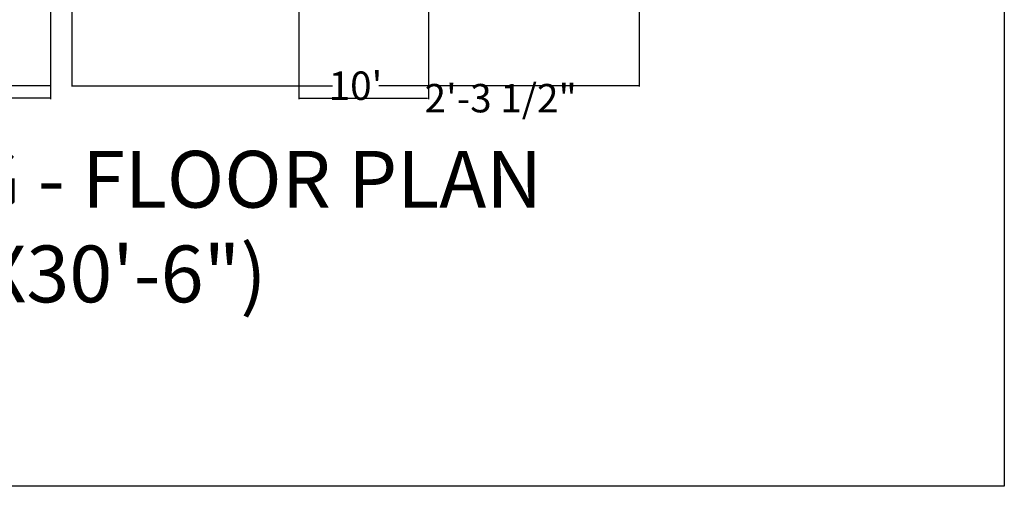
# Model space of a CAD drawing. Units: inches. Extents: x 958 to 1375, y 3152 to 3689.
# Tile 2 of 8: x 1167 to 1375, y 3152 to 3251. Entities that reach past the tile are written whole.
import ezdxf

# ---------------------------------------------------------------- set-up
doc = ezdxf.new("R2010")
doc.units = ezdxf.units.IN
doc.header["$MEASUREMENT"] = 0
doc.layers.add('A-ANNO-DIMS', color=2, linetype='Continuous', lineweight=18)
doc.layers.add('A-ANNO-TTLB', color=7, linetype='Continuous', lineweight=25)
doc.styles.get("Standard").update_dxf_attribs({"font": 'arial.ttf'})
doc.dimstyles.get("Standard").update_dxf_attribs({"dimtxt": 6, "dimasz": 0.18, "dimexe": 0.18, "dimexo": 0.0625, "dimgap": 0.09, "dimtad": 0, "dimtih": 1, "dimtoh": 1, "dimdec": 1, "dimzin": 0, "dimdsep": 46, "dimlunit": 3, "dimtxsty": 'Standard', "dimcen": 0.09, "dimadec": 0, "dimazin": 0, "dimtfac": 1, "dimtdec": 1, "dimtofl": 0, "dimtmove": 0, "dimatfit": 3, "dimfxl": 1, "dimtolj": 1, "dimtzin": 0, "dimarcsym": 0})

# ---------------------------------------------------------------- blocks, each defined once
blk = doc.blocks.new('*D9')
at = {"layer": 'A-ANNO-DIMS', "color": 0, "lineweight": -2, "transparency": 16777216}
for p, q in [((1177.7, 3257.97), (1177.7, 3236.74)), ((1297.7, 3257.97), (1297.7, 3236.74)), ((1177.88, 3236.92), (1232.8, 3236.92)), ((1297.52, 3236.92), (1242.6, 3236.92))]:
    blk.add_line(p, q, dxfattribs=at)
at = {"layer": 'A-ANNO-DIMS', "color": 0, "transparency": 16777216}
for points in [[(1177.88, 3236.95), (1177.88, 3236.89), (1177.7, 3236.92)], [(1297.52, 3236.95), (1297.52, 3236.89), (1297.7, 3236.92)]]:
    blk.add_solid(points, dxfattribs=at)
at = {"layer": 'Defpoints', "color": 0, "transparency": 16777216}
for p in [(1177.7, 3258.03), (1297.7, 3258.03), (1177.7, 3236.92)]:
    blk.add_point(p, dxfattribs=at)
at = {"layer": 'A-ANNO-DIMS', "color": 0, "transparency": 16777216, "insert": (1237.7, 3236.92), "char_height": 6, "attachment_point": 5}
blk.add_mtext("\\A1;10'", dxfattribs=at)
blk = doc.blocks.new('*D10')
at = {"layer": 'A-ANNO-DIMS', "color": 0, "lineweight": -2, "transparency": 16777216}
for p, q in [((1053.2, 3257.97), (1053.2, 3236.74)), ((1173.2, 3257.97), (1173.2, 3236.74)), ((1053.38, 3236.92), (1108.3, 3236.92)), ((1173.02, 3236.92), (1118.1, 3236.92))]:
    blk.add_line(p, q, dxfattribs=at)
at = {"layer": 'A-ANNO-DIMS', "color": 0, "transparency": 16777216}
for points in [[(1053.38, 3236.95), (1053.38, 3236.89), (1053.2, 3236.92)], [(1173.02, 3236.95), (1173.02, 3236.89), (1173.2, 3236.92)]]:
    blk.add_solid(points, dxfattribs=at)
at = {"layer": 'Defpoints', "color": 0, "transparency": 16777216}
for p in [(1053.2, 3258.03), (1173.2, 3258.03), (1173.2, 3236.92)]:
    blk.add_point(p, dxfattribs=at)
at = {"layer": 'A-ANNO-DIMS', "color": 0, "transparency": 16777216, "insert": (1113.2, 3236.92), "char_height": 6, "attachment_point": 5}
blk.add_mtext("\\A1;10'", dxfattribs=at)
blk = doc.blocks.new('*D49')
at = {"layer": 'A-ANNO-DIMS', "color": 0, "lineweight": -2, "transparency": 16777216}
for p, q in [((1225.7, 3386.97), (1225.7, 3234.1)), ((1253.12, 3386.97), (1253.12, 3234.1)), ((1225.88, 3234.28), (1252.94, 3234.28)), ((1253.12, 3234.28), (1253.3, 3234.28))]:
    blk.add_line(p, q, dxfattribs=at)
at = {"layer": 'A-ANNO-DIMS', "color": 0, "transparency": 16777216}
for points in [[(1225.88, 3234.31), (1225.88, 3234.25), (1225.7, 3234.28)], [(1252.94, 3234.31), (1252.94, 3234.25), (1253.12, 3234.28)]]:
    blk.add_solid(points, dxfattribs=at)
at = {"layer": 'Defpoints', "color": 0, "transparency": 16777216}
for p in [(1225.7, 3387.03), (1253.12, 3387.03), (1253.12, 3234.28)]:
    blk.add_point(p, dxfattribs=at)
at = {"layer": 'A-ANNO-DIMS', "color": 0, "transparency": 16777216, "insert": (1268.4, 3234.28), "char_height": 6, "attachment_point": 5}
blk.add_mtext('\\A1;2\'-3 1/2"', dxfattribs=at)
blk = doc.blocks.new('*D60')
at = {"layer": 'A-ANNO-DIMS', "color": 0, "lineweight": -2, "transparency": 16777216}
for p, q in [((1135.31, 3386.97), (1135.31, 3234.1)), ((1173.2, 3386.97), (1173.2, 3234.1)), ((1135.49, 3234.28), (1146.19, 3234.28)), ((1173.02, 3234.28), (1162.32, 3234.28))]:
    blk.add_line(p, q, dxfattribs=at)
at = {"layer": 'A-ANNO-DIMS', "color": 0, "transparency": 16777216}
for points in [[(1135.49, 3234.31), (1135.49, 3234.25), (1135.31, 3234.28)], [(1173.02, 3234.31), (1173.02, 3234.25), (1173.2, 3234.28)]]:
    blk.add_solid(points, dxfattribs=at)
at = {"layer": 'Defpoints', "color": 0, "transparency": 16777216}
for p in [(1135.31, 3387.03), (1173.2, 3387.03), (1173.2, 3234.28)]:
    blk.add_point(p, dxfattribs=at)
at = {"layer": 'A-ANNO-DIMS', "color": 0, "transparency": 16777216, "insert": (1154.25, 3234.28), "char_height": 6, "attachment_point": 5}
blk.add_mtext('\\A1;3\'-2"', dxfattribs=at)

msp = doc.modelspace()

# ---------------------------------------------------------------- linework, layer by layer
at = {"layer": 'A-ANNO-TTLB'}
msp.add_lwpolyline([(958.44, 3689.37), (1374.91, 3689.37), (1374.91, 3152.28), (958.44, 3152.28)], close=True, dxfattribs=at)

# ---------------------------------------------------------------- texts
at = {"layer": 'A-ANNO-TTLB', "insert": (1065.83, 3223.15), "char_height": 12, "attachment_point": 1}
msp.add_mtext_dynamic_manual_height_columns('PROPOSED G - FLOOR PLAN\\P         (21\'-10"X30\'-6")', width=421.2695, gutter_width=1, heights=[0], dxfattribs=at)

# ---------------------------------------------------------------- dimensions: what is measured, and where the dimension line sits
at = {"layer": 'A-ANNO-DIMS'}
for base, p1, p2, override, picture, middle in [((1173.2, 3234.28), (1135.31, 3387.03), (1173.2, 3387.03), {"dimdec": 1, "dimlfac": 1, "dimrnd": 0, "dimzin": 1, "dimdsep": 46, "dimlunit": 4, "dimfrac": 2}, '*D60', (1154.25, 3234.28)), ((1253.12, 3234.28), (1225.7, 3387.03), (1253.12, 3387.03), {"dimdec": 1, "dimlfac": 1, "dimrnd": 0, "dimzin": 1, "dimdsep": 46, "dimlunit": 4, "dimfrac": 2}, '*D49', (1268.4, 3234.28)), ((1173.2, 3236.92), (1053.2, 3258.03), (1173.2, 3258.03), {"dimclrd": 0, "dimclre": 0, "dimclrt": 0}, '*D10', (1113.2, 3236.92)), ((1177.7, 3236.92), (1297.7, 3258.03), (1177.7, 3258.03), {"dimclrd": 0, "dimclre": 0, "dimclrt": 0}, '*D9', (1237.7, 3236.92))]:
    dim = msp.add_linear_dim(base=base, p1=p1, p2=p2, dimstyle='Standard', override=override, dxfattribs=at)
    dim.commit()
    dim.dimension.update_dxf_attribs({"geometry": picture, "text_midpoint": middle})

doc.saveas('drawing.dxf')
